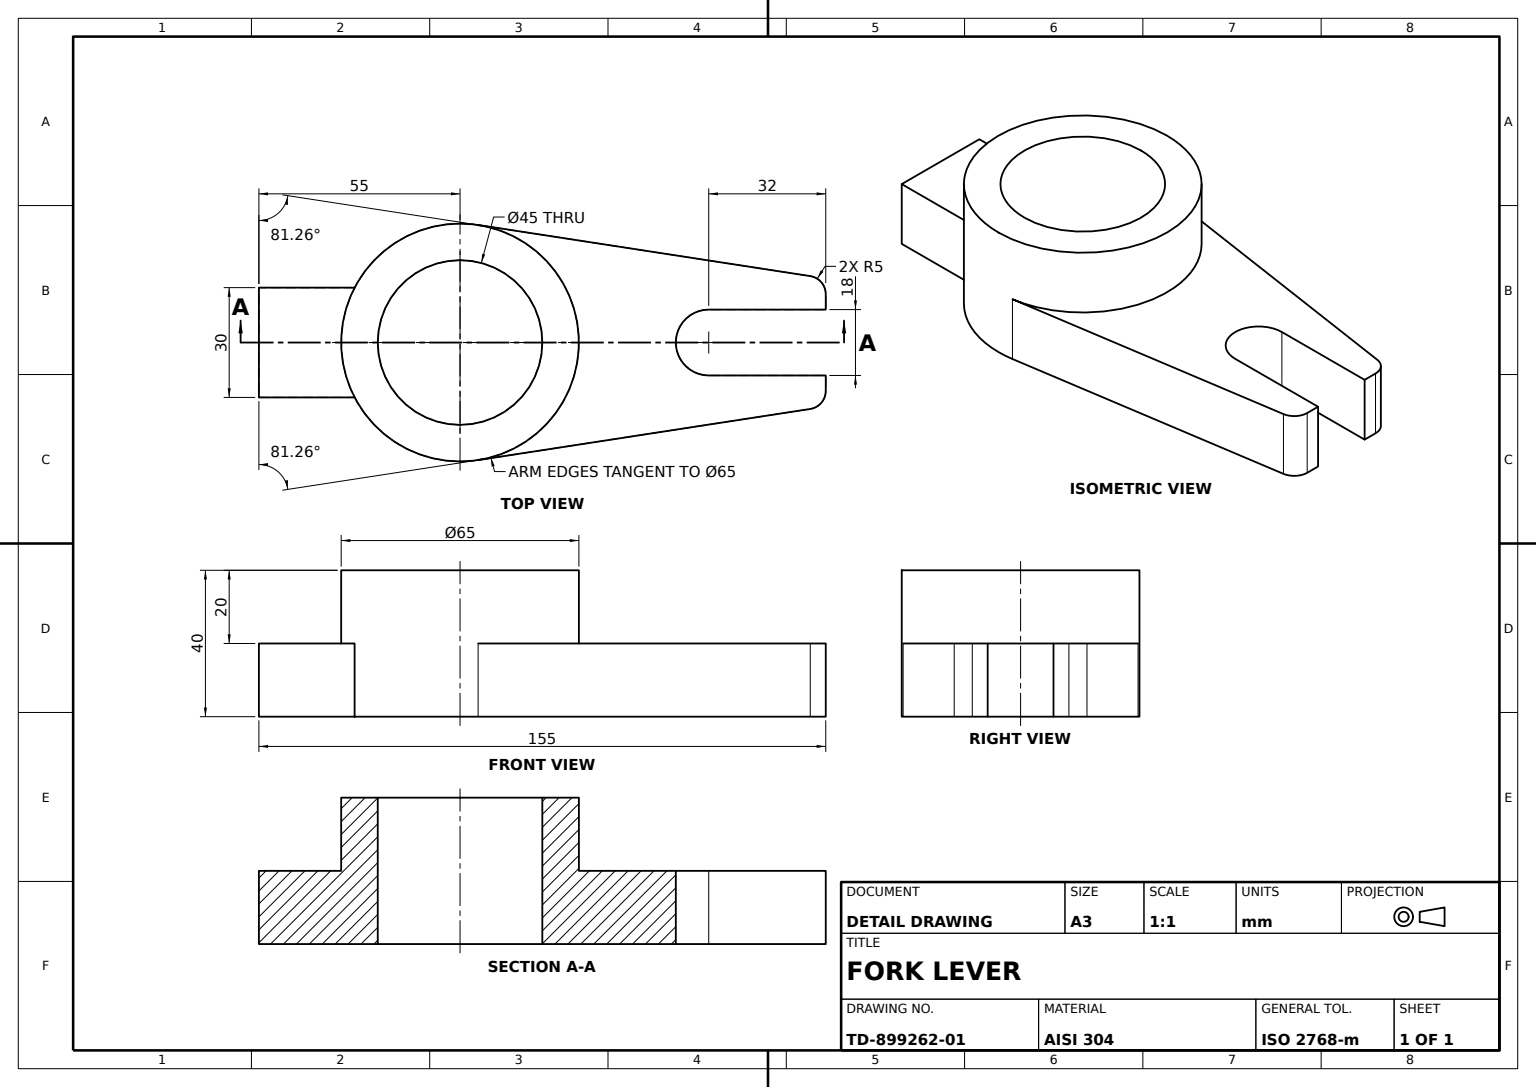
from build123d import *

# Parameters (mm, degrees)
HUB_RING_SKETCH_R     = 32.5
HUB_RING_SKETCH_R_2   = 22.5
HUB_RING_65X_45_DEPTH = 20
FORK_ARM_DEPTH        = 20
REAR_TAB_DEPTH        = 20


with BuildPart() as part:
    # Hub Ring Sketch → Hub Ring Ø65xØ45 (new, symmetric)
    with BuildSketch(Plane(origin=(0, 0, 0), x_dir=(1, 0, 0), z_dir=(0, 1, 0))):
        with Locations(Location((0, 0, 0), (0, 0, 270))):
            Circle(HUB_RING_SKETCH_R)
        with Locations(Location((0, 0, 0), (0, 0, 270))):
            Circle(HUB_RING_SKETCH_R_2, mode=Mode.SUBTRACT)
    extrude(amount=HUB_RING_65X_45_DEPTH, both=True)

    # Fork Arm Sketch → Fork Arm (add)
    with BuildSketch(Plane(origin=(0, 0, 0), x_dir=(1, 0, 0), z_dir=(0, 1, 0))):
        with BuildLine():
            Line((95.760171689, 18.152180955), (4.941115981, 32.122194397))
            ThreePointArc((4.941115981, 32.122194397), (32.5, 0), (4.941115981, -32.122194397))
            Line((4.941115981, -32.122194397), (95.760171689, -18.152180955))
            ThreePointArc((95.760171689, -18.152180955), (98.794789747, -16.466003095), (100, -13.210304894))
            Line((100, -13.210304894), (100, -9))
            Line((100, -9), (68, -9))
            ThreePointArc((68, -9), (59, 0), (68, 9))
            Line((68, 9), (100, 9))
            Line((100, 9), (100, 13.210304894))
            ThreePointArc((100, 13.210304894), (98.794789747, 16.466003095), (95.760171689, 18.152180955))
        make_face()
    extrude(amount=-FORK_ARM_DEPTH)

    # Rear Tab Sketch → Rear Tab (add)
    with BuildSketch(Plane(origin=(0, 0, 0), x_dir=(1, 0, 0), z_dir=(0, 1, 0))):
        with BuildLine():
            Line((-28.831406487, 15), (-55, 15))
            Line((-55, 15), (-55, -15))
            Line((-55, -15), (-28.831406487, -15))
            ThreePointArc((-28.831406487, -15), (-32.5, 0), (-28.831406487, 15))
        make_face()
    extrude(amount=-REAR_TAB_DEPTH)


solid = part.part
